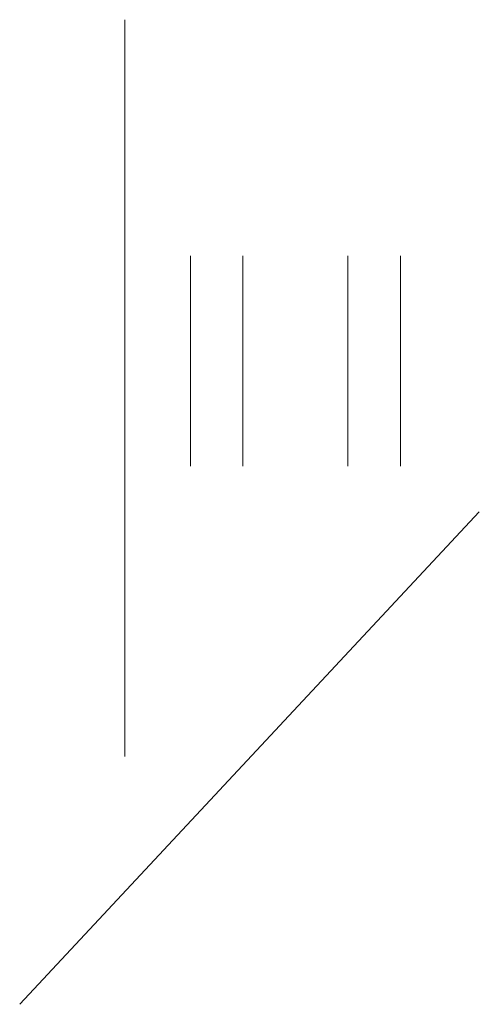
# Model space of a CAD drawing. Units: millimetres. Extents: x 449 to 519, y 951 to 1101.
import ezdxf

# ---------------------------------------------------------------- set-up
doc = ezdxf.new("R2010")
doc.units = ezdxf.units.MM
doc.layers.add('M-CONS', color=8, linetype='Continuous', lineweight=13)

msp = doc.modelspace()

# ---------------------------------------------------------------- linework, layer by layer
at = {"layer": 'M-CONS'}
for p, q in [((464.64, 988.75, 87.51), (464.64, 1101.01, 16)), ((474.64, 1033.01, 16), (474.64, 1065.01, 16)), ((482.64, 1065.01, 16), (482.64, 1033.01, 16)), ((498.64, 1033.01, 16), (498.64, 1065.01, 16)), ((506.64, 1065.01, 16), (506.64, 1033.01, 16)), ((518.64, 1026.01, 16), (448.64, 951.01, 16))]:
    msp.add_line(p, q, dxfattribs=at)

doc.saveas('drawing.dxf')
